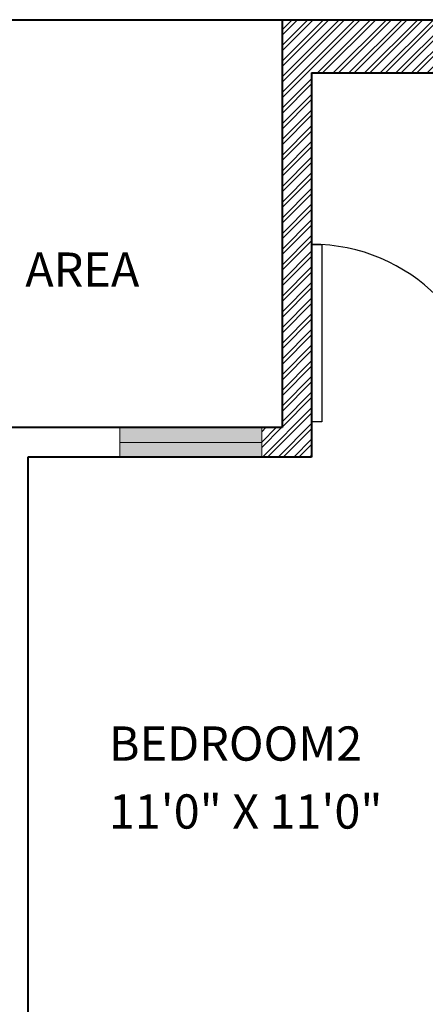
# Model space of a CAD drawing. Units: inches. Extents: x 528 to 2520, y -151 to 1354.
# Tile 37 of 41: x 2315 to 2383, y 731 to 898. Entities that reach past the tile are written whole.
import ezdxf

# ---------------------------------------------------------------- set-up
doc = ezdxf.new("R2010")
doc.units = ezdxf.units.IN
doc.header["$MEASUREMENT"] = 0
for name, color, linetype, lineweight in [('A-AREA-IDEN', 7, 'Continuous', 18), ('A-Door', 150, 'Continuous', 25), ('A-WALL-PATT', 6, 'Continuous', 13), ('walls', 7, 'Continuous', 40), ('WINDOWS', 2, 'Continuous', 20)]:
    doc.layers.add(name, color=color, linetype=linetype, lineweight=lineweight)
doc.layers.add('A-GLAZ-PATT', color=152, linetype='Continuous', lineweight=13, true_color=0x2776bb)
doc.styles.get("Standard").update_dxf_attribs({"font": 'arial.ttf'})

# ---------------------------------------------------------------- blocks, each defined once
blk = doc.blocks.new('DOOR-SWING-30')
for p, q in [((0, 6), (0, 0)), ((30, 6), (30, 0))]:
    blk.add_line(p, q)
blk.add_lwpolyline([(0, 6), (0, 36), (1.75, 36), (1.75, 6)], close=True)
blk.add_arc((0, 6), 30, 0, 90)
blk = doc.blocks.new('WINDOW-24x5-PLAN')
for p, q in [((0, 5), (24, 5)), ((24, 0), (24, 5)), ((0, 2.5), (24, 2.5))]:
    blk.add_line(p, q)
blk.add_lwpolyline([(0, 5), (24, 5), (24, 0), (0, 0)], close=True)

msp = doc.modelspace()

# ---------------------------------------------------------------- hatches: boundary and pattern name
at = {"layer": 'A-GLAZ-PATT'}
h = msp.add_hatch(color=256, dxfattribs=at)
h.dxf.hatch_style = 1
h.paths.add_polyline_path([(2355.58, 828.94), (2331.58, 828.94), (2331.58, 826.44), (2355.58, 826.44)])
h.paths.add_polyline_path([(2355.58, 826.44), (2331.58, 826.44), (2331.58, 823.94), (2355.58, 823.94)])
at = {"layer": 'A-WALL-PATT'}
h = msp.add_hatch(dxfattribs=at)
h.set_pattern_fill('ANSI32', color=256, scale=5)
h.set_pattern_definition([(45, (1571.3155, -419.1643), (-1.3258252, 1.3258252), []), (45, (1572.1993, -419.1643), (-1.3258252, 1.3258252), [])])
h.paths.add_polyline_path([(2167.01, 744.69), (2158.01, 744.69), (2158.01, 549.94), (2169.56, 549.94), (2174.56, 549.94), (2174.56, 554.94), (2167.01, 554.94), (2167.01, 662.94), (2263.01, 662.94), (2263.01, 667.94), (2263.01, 686.94), (2269.01, 686.94), (2269.01, 691.94), (2258.01, 691.94), (2258.01, 667.94), (2167.01, 667.94)])
h.paths.add_polyline_path([(2260.02, 554.94), (2222.56, 554.94), (2222.56, 549.94), (2260.02, 549.94)])
h.paths.add_polyline_path([(2457.01, 752.2), (2448.01, 752.2), (2448.01, 691.94), (2358.01, 691.94), (2358.01, 686.94), (2448.01, 686.94), (2448.01, 554.94), (2358.01, 554.94), (2358.01, 549.94), (2448.01, 549.94), (2448.01, 405.94), (2406.01, 405.94), (2406.01, 396.94), (2457.01, 396.94)])
h.paths.add_polyline_path([(2457.01, 897.94), (2447.97, 897.94), (2447.97, 888.94), (2448.01, 888.94), (2448.01, 828.94), (2394.01, 828.94), (2394.01, 823.94), (2448.01, 823.94), (2448.01, 800.2), (2457.01, 800.2)])
h.paths.add_polyline_path([(2423.97, 897.94), (2359.01, 897.94), (2359.01, 828.94), (2355.58, 828.94), (2355.58, 823.94), (2364.01, 823.94), (2364.01, 829.94), (2364.01, 888.94), (2423.97, 888.94)])
h.paths.add_polyline_path([(2256.01, 897.94), (2191.01, 897.94), (2191.01, 888.94), (2251.01, 888.94), (2251.01, 828.94), (2251.01, 823.94), (2256.01, 823.94), (2256.01, 829.08)])
h.paths.add_polyline_path([(2167.01, 888.94), (2167.01, 897.94), (2158.01, 897.94), (2158.01, 792.69), (2167.01, 792.69), (2167.01, 823.94), (2221.01, 823.94), (2221.01, 828.94), (2167.01, 828.94)])
h.paths.add_polyline_path([(2316.01, 549.94), (2316.01, 554.94), (2296.02, 554.94), (2296.02, 549.94), (2311.01, 549.94), (2311.01, 455.12), (2316.01, 455.12)])
h.paths.add_polyline_path([(2311.01, 549.94), (2299.01, 549.94), (2299.01, 545.95), (2302.05, 545.95), (2302.05, 542.51), (2305.75, 542.51), (2305.75, 538.08), (2311.01, 538.08)], flags=17)
h.paths.add_polyline_path([(2358.01, 405.94), (2316.01, 405.94), (2316.01, 413.12), (2311.01, 413.12), (2311.01, 396.94), (2358.01, 396.94)])

# ---------------------------------------------------------------- linework, layer by layer
at = {"layer": 'walls'}
for p, q in [((2256.01, 897.94), (2359.01, 897.94)), ((2359.01, 897.94), (2359.01, 828.94)), ((2359.01, 897.94), (2457.01, 897.94)), ((2364.01, 888.94), (2364.01, 828.94)), ((2364.01, 888.94), (2448.01, 888.94)), ((2359.01, 828.94), (2292.01, 828.94)), ((2364.01, 828.94), (2364.01, 823.94)), ((2316.01, 823.94), (2316.01, 691.94)), ((2364.01, 823.94), (2316.01, 823.94))]:
    msp.add_line(p, q, dxfattribs=at)

# ---------------------------------------------------------------- block references
at = {"layer": 'A-Door'}
msp.add_blockref('DOOR-SWING-30', (2364.01, 823.94), dxfattribs=at)
at = {"layer": 'WINDOWS'}
msp.add_blockref('WINDOW-24x5-PLAN', (2331.58, 823.94), dxfattribs=at)

# ---------------------------------------------------------------- texts
at = {"layer": 'A-AREA-IDEN'}
for s, height, p in [('OPEN AREA', 5.793, (2292.6, 852.77)), ('BEDROOM2', 5.793, (2329.73, 772.61)), ('11\'0" X 11\'0"', 5.7926, (2329.73, 761.12))]:
    msp.add_text(s, height=height, dxfattribs=at).set_placement(p)

doc.saveas('drawing.dxf')
